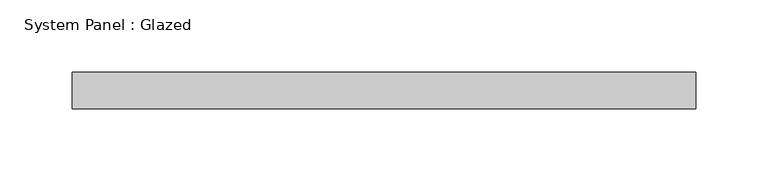
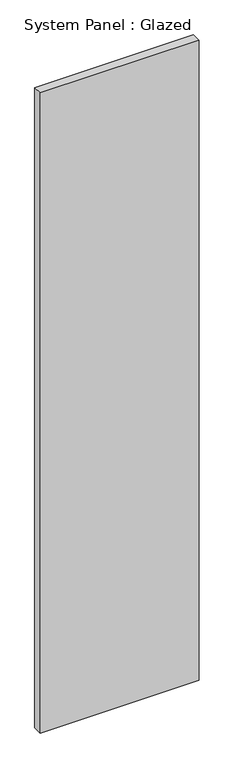
"""IFC4 building model written with IfcOpenShell, lengths in millimetres: plate geometry, System Panel : Glazed."""

from ifc_helpers import new_model, si_unit, origin, origin_with_axes, place, context, project, spatial, polyline, outline, extrude, source, transform, mapped, element, save


def system_panel_glazed_f7c25410(model_context):
    return source(origin(), model_context, "Body", "SweptSolid", [
        extrude(outline(polyline([(215.9, 19.05), (-215.9, 19.05), (-215.9, 44.45), (215.9, 44.45), (215.9, 19.05)])), origin_with_axes(), (0.0, 0.0, 1.0), 1837.4891744),
    ])


if __name__ == "__main__":
    model = new_model("IFC4")
    model_context = context("Model", 3, world=origin())
    ifc_project = project(units=[si_unit("LENGTHUNIT", "METRE", prefix="MILLI")], contexts=[model_context])
    site = spatial("IfcSite", under=ifc_project)
    building = spatial("IfcBuilding", under=site)
    placement = place(None, origin())
    system_panel_glazed_shape = system_panel_glazed_f7c25410(model_context)
    element("IfcPlate", 1, ObjectType="System Panel : Glazed", at=placement, inside=building, context=model_context, shape_type="MappedRepresentation", body=[
        mapped(system_panel_glazed_shape, transform((0.0, 0.0, 0.0), x_axis=(1.0, 0.0, 0.0), y_axis=(0.0, 1.0, 0.0), z_axis=(0.0, 0.0, 1.0))),
    ])
    save(model, "model.ifc")

# Revit data of these elements
# Type "System Panel : Glazed"
#   Construction Type Id = "GSP4R"
#   Analytic Construction = "1/8 in Pilkington single glazing"
#   Visual Light Transmittance = 0.9
#   Solar Heat Gain Coefficient = 0.86
#   Heat Transfer Coefficient (U) = 1.18115 BTU/(h·ft²·°F)
#   Define Thermal Properties by = 1
# Element 1 (IfcPlate, "System Panel : Glazed")
#   Materials on its faces: "Glass"
# Materials
#   "Glass": class "Glass", colour RGB 0 128 192, transparency 0.75, Description = "Soda Lime Glass", Cost = 0
